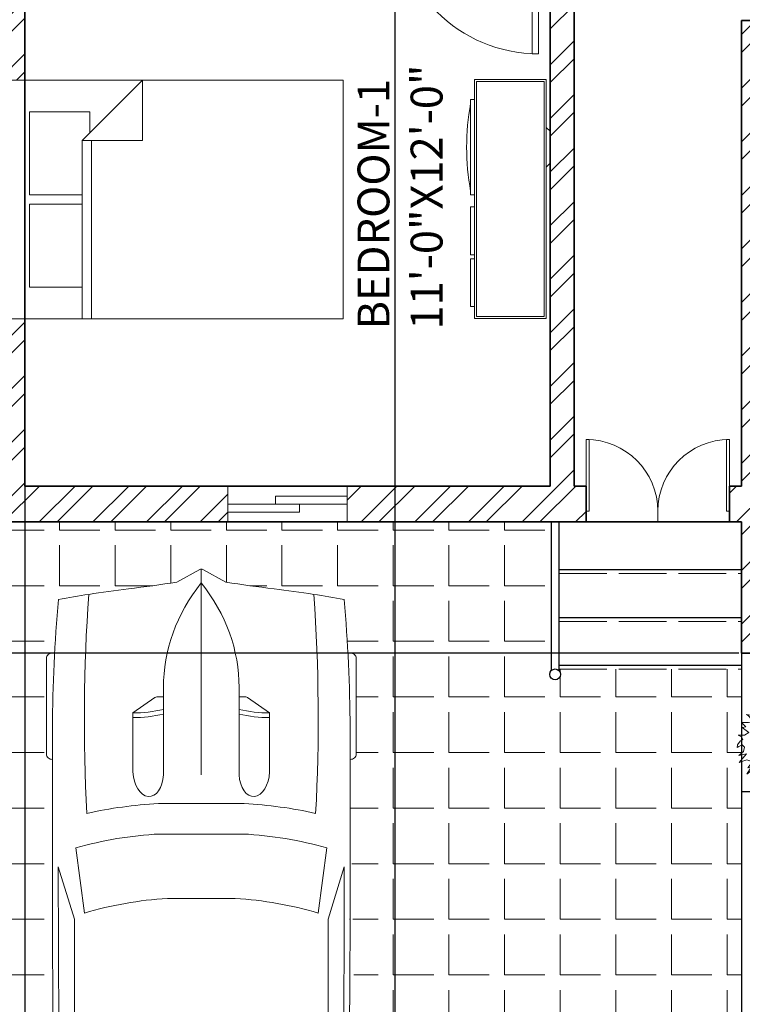
# Model space of a CAD drawing. Units: inches. Extents: x 889 to 1572, y 7262 to 8387.
# Tile 1 of 8: x 1024 to 1205, y 7495 to 7742. Entities that reach past the tile are written whole.
import ezdxf

# ---------------------------------------------------------------- set-up
doc = ezdxf.new("R2010")
doc.units = ezdxf.units.IN
doc.linetypes.add('ACAD_ISO02W100', pattern=[15, 12, -3])
for name, color, linetype, lineweight in [('A-ANNO-DIMS', 2, 'Continuous', 18), ('A-AREA-IDEN', 7, 'Continuous', 18), ('A-DOOR', 4, 'Continuous', 18), ('A-FLOR-STRS', 7, 'Continuous', 25), ('A-FURN', 8, 'Continuous', 18), ('A-STRS-HIDN', 8, 'ACAD_ISO02W100', 13), ('A-WALL', 7, 'Continuous', 35), ('A-WALL-PATT', 252, 'Continuous', 13), ('C-SITE', 7, 'Continuous', 30), ('C-VEHI', 8, 'Continuous', 18), ('L-PLNT', 94, 'Continuous', 13), ('L-PVMT-PATT', 252, 'Continuous', 13)]:
    doc.layers.add(name, color=color, linetype=linetype, lineweight=lineweight)
doc.layers.add('A-GLAZ', color=244, linetype='Continuous', lineweight=18, true_color=0x991b1e)
doc.styles.get("Standard").update_dxf_attribs({"font": 'arial.ttf'})
doc.dimstyles.new('ISO-25', dxfattribs={"dimtxt": 9, "dimasz": 2.5, "dimexe": 1.25, "dimexo": 0.625, "dimtad": 1, "dimlunit": 3, "dimtxsty": 'Standard', "dimcen": 2.5, "dimadec": 0, "dimazin": 0, "dimtfac": 1, "dimtmove": 0, "dimatfit": 3, "dimfxl": 1, "dimarcsym": 0})

# ---------------------------------------------------------------- blocks, each defined once
blk = doc.blocks.new('*U2')
for p, q in [((0, 0), (-1e-16, -5.999999999999999)), ((40, -6e-16), (40, -6))]:
    blk.add_line(p, q)
blk.add_lwpolyline([(0, 0), (5.6e-15, 40), (1.750000000000007, 40), (1.749999999999998, -7e-16)], close=True)
blk.add_arc((0, 0), 40, 0, 90)
blk = doc.blocks.new('*U3')
for p, q in [((0, 0), (0, -5.999999999999999)), ((-40, -6e-16), (-40, -6))]:
    blk.add_line(p, q)
blk.add_lwpolyline([(0, 0), (-7.1e-15, 40), (-1.750000000000007, 40), (-1.75, -7e-16)], close=True)
blk.add_arc((0, 0), 40, 90, 180)
blk = doc.blocks.new('*U5')
for p, q in [((-40, -1.47e-14), (-40, 5.999999999999984)), ((0, 0), (0, 5.999999999999999))]:
    blk.add_line(p, q)
blk.add_lwpolyline([(0, 0), (7.1e-15, -40), (-1.749999999999992, -40), (-1.75, -1e-16)], close=True)
blk.add_arc((0, 0), 40, 180, 270)
blk = doc.blocks.new('Bed - Queen')
for p, q in [((0, -80.00003000000002), (0, 0)), ((0, 0), (59.99998999999999, 0)), ((59.99998999999999, 0), (59.99998999999999, -80.00003000000002)), ((7.99999, -1.200000000000017), (28.79998, -1.200000000000017)), ((7.99999, -14.4), (7.99999, -1.200000000000017)), ((28.79998, -1.200000000000017), (28.79998, -14.4)), ((31.19999, -1.200000000000017), (51.99999000000001, -1.200000000000017)), ((31.19999, -14.4), (31.19999, -1.200000000000017)), ((51.99999000000001, -1.200000000000017), (51.99999000000001, -16.4)), ((0, -14.4), (44.79999999999999, -14.4)), ((59.99998999999999, -29.60000000000001), (44.79999999999999, -14.4)), ((44.79999999999999, -14.4), (44.79999999999999, -29.60000000000001)), ((44.79999999999999, -16.80000000000001), (0, -16.80000000000001)), ((51.99999000000001, -16.4), (46.79936, -16.4)), ((44.79999999999999, -29.60000000000001), (59.99998999999999, -29.60000000000001)), ((59.99998999999999, -80.00003000000002), (0, -80.00003000000002))]:
    blk.add_line(p, q)
blk = doc.blocks.new('Entertainment Center')
for p, q in [((-4, 0), (-5, -1)), ((4, 0), (-4, 0)), ((5, -1), (4, 0)), ((-17, -19.00000000000003), (-17, -1)), ((-17, -1), (43, -1)), ((-16.5, -18.50000000000003), (-16.5, -1.5)), ((-16.5, -1.5), (42.5, -1.5)), ((42.5, -1.5), (42.5, -18.50000000000003)), ((43, -1), (43, -19.00000000000003)), ((43, -19.00000000000003), (-17, -19.00000000000003)), ((42.5, -18.50000000000003), (-16.5, -18.50000000000003)), ((-12, -20.00000000000003), (-12, -19.00000000000003)), ((12, -19.00000000000003), (12, -20.00000000000003)), ((15, -20.00000000000003), (15, -19.00000000000003)), ((27, -19.00000000000003), (27, -20.00000000000003)), ((28, -20.00000000000003), (28, -19.00000000000003)), ((40, -19.00000000000003), (40, -20.00000000000003)), ((12, -20.00000000000003), (-12, -20.00000000000003)), ((27, -20.00000000000003), (15, -20.00000000000003)), ((40, -20.00000000000003), (28, -20.00000000000003))]:
    blk.add_line(p, q)
blk.add_arc((0, 40), 61.0000000000039, 259.6111000000045, 280.3888999999955)
blk = doc.blocks.new('*U19')
for points in [[(0, 60.6400000000001), (-3.051000000000385, 56.23799999999983), (-4.196000000000367, 52.81500000000005), (-5.33999999999969, 47.92499999999995), (-6.10299999999961, 45.96900000000005), (-11.0619999999999, 50.85899999999992), (-18.69100000000026, 52.32600000000002), (-20.98000000000002, 47.43600000000014), (-20.2170000000001, 43.52399999999988), (-20.5979999999995, 39.61100000000011), (-25.93899999999985, 43.03500000000008), (-27.84600000000001, 49.39200000000005), (-33.18600000000015, 52.32600000000002), (-30.51600000000008, 47.43600000000014), (-31.279, 43.03500000000008), (-30.13499999999976, 38.14400000000001), (-33.56799999999976, 35.21000000000004), (-40.8149999999996, 36.67700000000014), (-49.20799999999963, 38.14400000000001), (-46.91899999999987, 36.67700000000014), (-42.34100000000035, 31.78700000000004), (-42.34100000000035, 28.36400000000003), (-46.53699999999981, 27.38599999999997), (-55.69200000000001, 27.38599999999997), (-49.9699999999998, 22.00600000000008), (-54.54799999999977, 21.02799999999979), (-46.15599999999995, 14.67100000000005), (-51.4960000000001, 11.24799999999982), (-59.88799999999992, 11.24799999999982), (-55.69200000000001, 8.802999999999884), (-53.78499999999985, 5.380000000000109), (-57.21799999999984, 3.423000000000001), (-60.65100000000029, -1.467000000000098), (-61.0329999999999, -4.889999999999872), (-59.125, -3.422999999999774), (-54.54799999999977, -1.467000000000098), (-51.4960000000001, -4.401000000000067), (-53.02199999999993, -10.269), (-59.125, -15.16000000000008), (-49.20799999999963, -13.20399999999995), (-58.36200000000008, -24.45100000000002), (-48.44499999999971, -21.02799999999979), (-43.48600000000033, -22.49499999999989), (-43.10400000000027, -25.91799999999989), (-47.29999999999972, -31.29799999999978), (-43.10400000000027, -30.31999999999994), (-48.44499999999971, -39.61100000000011), (-38.52700000000004, -31.78700000000004), (-40.8149999999996, -36.18799999999988), (-32.42299999999977, -37.16599999999994), (-33.56799999999976, -43.52299999999991), (-35.47499999999991, -49.39200000000005), (-28.60899999999992, -44.99000000000001), (-23.64999999999964, -46.45700000000011), (-22.12400000000025, -51.83699999999999), (-21.74299999999949, -57.70499999999993), (-19.07299999999986, -52.32600000000002), (-15.63900000000012, -51.83699999999999), (-12.58799999999974, -58.68299999999976), (-11.0619999999999, -54.77099999999996), (-6.865999999999985, -49.39200000000005), (-6.865999999999985, -53.30399999999986), (-4.958999999999832, -48.41399999999999), (-1.907000000000152, -61.61700000000019), (-1.144000000000232, -51.34799999999995), (4.577999999999974, -59.17200000000002), (5.340999999999894, -54.28200000000015), (9.91800000000012, -56.72700000000009), (12.20700000000033, -60.63899999999989), (12.97000000000025, -47.92499999999995), (14.87700000000041, -44.50099999999998), (17.54700000000048, -47.43600000000014), (19.45500000000038, -52.81500000000005), (22.88799999999992, -60.63899999999989), (21.74299999999994, -49.39200000000005), (23.65000000000009, -46.45700000000011), (29.75399999999991, -47.92499999999995), (35.09400000000005, -52.32600000000002), (37.00099999999975, -53.79299999999989), (33.18700000000035, -46.45700000000011), (32.04200000000037, -41.567), (35.09400000000005, -39.12200000000007), (43.86799999999993, -40.58899999999994), (47.68200000000024, -42.05600000000004), (43.10500000000001, -36.18799999999988), (43.10500000000001, -33.74299999999994), (46.53800000000001, -31.29799999999978), (50.35200000000031, -32.76499999999987), (46.91899999999987, -26.40700000000015), (55.69300000000021, -22.49499999999989), (60.6520000000005, -22.98399999999992), (66.3739999999998, -22.00600000000008), (59.88899999999967, -20.04999999999995), (54.16700000000037, -18.09399999999982), (51.87800000000016, -15.64899999999989), (49.58899999999994, -12.22499999999991), (51.4970000000003, -10.269), (57.98099999999976, -9.779999999999973), (63.32200000000011, -7.335000000000036), (64.4659999999999, -2.933999999999969)], [(64.84799999999996, -2.933999999999969), (59.50700000000051, -5.378999999999905), (56.45600000000013, -4.401000000000067), (51.87800000000016, -2.444999999999936), (52.26000000000022, 0.9779999999998381), (55.31100000000015, 3.912000000000034), (59.88899999999967, 5.868999999999914), (62.94000000000005, 11.24799999999982), (58.36300000000028, 10.26999999999998), (54.54800000000023, 10.26999999999998), (51.11500000000024, 11.24799999999982), (53.7850000000003, 15.64899999999989), (57.98099999999976, 18.09400000000005), (60.6520000000005, 19.56100000000015), (56.07399999999961, 19.56100000000015), (51.11500000000024, 17.60500000000002), (46.53800000000001, 19.07200000000011), (46.15599999999995, 22.49600000000009), (49.58899999999994, 27.38599999999997), (52.26000000000022, 34.72100000000001), (49.58899999999994, 33.74299999999994), (44.24899999999979, 30.31999999999994), (41.19700000000011, 32.27600000000007), (41.57899999999972, 37.65499999999998), (43.86799999999993, 42.54600000000005), (43.10500000000001, 46.94700000000011), (40.05299999999988, 44.01299999999991), (36.23800000000028, 40.58899999999994), (33.56800000000021, 42.05700000000024), (33.95000000000027, 45.96900000000005), (35.47600000000012, 52.81500000000005), (31.2800000000002, 49.39200000000005), (26.70200000000022, 46.94700000000011), (28.22800000000007, 50.85899999999992), (28.60899999999992, 61.1289999999999), (24.79500000000007, 54.28200000000015), (18.69200000000046, 50.85899999999992), (17.92899999999963, 57.70600000000013), (12.97000000000025, 50.85899999999992), (7.248000000000047, 57.70600000000013), (5.340999999999894, 53.30399999999986), (0, 60.6400000000001)]]:
    blk.add_lwpolyline(points)
blk.add_lwpolyline([(0.3820000000005166, 1.95600000000013), (0, 0), (1.907000000000152, 0.4890000000000328), (2.288999999999759, 1.467000000000098)], close=True)
blk = doc.blocks.new('*U21')
for p, q in [((21.10406751471477, 37.40863046792069), (21.10406751471477, 36.83230215753705)), ((46.55368679439944, 38.88847654282876), (22.35054758993934, 38.88847654282876)), ((47.80016686962392, 37.39011648242055), (47.80016686962392, 37.40863046792069)), ((135.4513231603356, 37.07354110333037), (135.4513231603356, 37.40863046792069)), ((136.6978032355602, 38.88847654282876), (160.90094244002, 38.88847654282867)), ((162.1474225152445, 37.40863046792049), (162.1474225152445, 36.77402019194128)), ((87.98532186932616, 31.87120872459877), (74.75900729854769, 35.92175679182955)), ((134.313356548143, 35.6043097713567), (119.2882629232503, 31.77757799177584)), ((186.4728846989705, -33.49860931502491), (186.4728846989718, 33.49860931502465)), ((188.3990091454065, -32.75868627757393), (188.3990091454077, 32.75868627757058)), ((70.0302824853563, 31.53613089391356), (86.40615155322342, 29.35124891408057)), ((138.4228833961707, 29.35124891408074), (157.2465674415997, 29.35124891408074)), ((186.4728846989718, 29.35124891408083), (167.0083537481071, 29.35124891408083)), ((164.515393597658, 26.39155676426461), (164.5153935976578, -26.39155676426503)), ((32.26591480791686, 11.62530558863241), (36.12873726252356, 17.16961494239206)), ((36.12873726252356, 17.16961494239206), (50.93891189819171, 17.16961494239206)), ((32.12291633764599, 9.505833383620029), (32.12291633764599, 11.15369945057711)), ((58.9167604809788, -10.77488335095668), (58.9167604809788, 10.77488335095617)), ((66.55009204259746, -10.5288681329018), (66.55009204259746, 10.52886813290129)), ((186.4728846989718, -10.5288681329018), (186.4728846989718, 10.52886813290129)), ((29.77279020470884, 9.505833383620029), (51.68362801571248, 9.505833383620029)), ((82.73706193978568, 8.496039918672748), (82.73706193978568, -8.49603991867258)), ((3.266462181856987, 6.128290093440767), (0.1022408397004821, 0.4060708604429806)), ((-4.43e-14, -2.558e-13), (51.68362801571248, -2.558e-13)), ((0.1022408397004821, -0.4060708604432933), (3.266462181856987, -6.128290093441194)), ((29.77279020470884, -9.50583338362054), (51.68362801571248, -9.50583338362054)), ((32.12291633764599, -9.50583338362054), (32.12291633764599, -11.15369945057762)), ((32.26591480791686, -11.62530558863292), (36.12873726252356, -17.16961494239257)), ((36.12873726252356, -17.16961494239257), (50.93891189819171, -17.16961494239257)), ((86.40615155322318, -29.35124891408145), (70.03028248535594, -31.53613089391442)), ((157.2465674415997, -29.35124891408117), (138.4228833961707, -29.35124891408126)), ((167.008353748107, -29.35124891408126), (186.4728846989707, -29.35124891408108)), ((87.98532186932607, -31.87120872459903), (74.7590072985476, -35.92175679182964)), ((134.3133565481428, -35.60430977135721), (119.2882629232503, -31.77757799177618)), ((21.10406751471477, -37.4086304679212), (21.10406751471477, -36.83230215753756)), ((135.4513231603355, -37.07354110333088), (135.4513231603355, -37.4086304679212)), ((162.1474225152445, -37.408630467921), (162.1474225152445, -36.77402019194179)), ((46.55368679439944, -38.88847654282927), (22.35054758993934, -38.88847654282927)), ((47.80016686962392, -37.39011648242107), (47.80016686962392, -37.4086304679212)), ((136.6978032355602, -38.88847654282927), (160.9009424400199, -38.88847654282918))]:
    blk.add_line(p, q)
for centre, major_axis, ratio, start_param, end_param in [((41.19115208863305, -490.8631038926156), (1.294e-13, 528.2339998381949), 0.8423038695439741, 0.0028100083536837, 0.0755983031096952), ((22.35054758993934, 37.40863046792072), (2.08e-14, -1.479846074908118), 0.842303869543976, 3.141592653589776, 4.712388980384677), ((64.48199294511879, -10555.61767587835), (1.907644e-10, 10593.02630634627), 0.842303869543847, -0.0133969486112073, 0.0027970409639888), ((46.55368679439944, 37.40863046792072), (2.2e-14, 1.479846074908118), 0.8423038695439758, -1.570796326794884, 1.73e-14), ((136.6978032355602, 37.40863046792072), (2.357e-13, -1.479846074908118), 0.842303869543976, 3.141592653589603, 4.712388980384554), ((160.90094244002, 37.40863046792052), (5.59e-14, 1.479846074908118), 0.842303869543976, -1.570796326794865, 4.44e-14), ((180.6280394947615, 35.8381667808375), (7.4e-14, 2.219769112362114), 0.8423038695439693, -0.0130174256259048, 1.249894140392862), ((64.48199294754608, -10556.35759891604), (1.349839377e-06, 10595.3130398087), 0.8423038681351469, -0.0133969484821159, -0.0130174254969711), ((183.9799245485216, 32.75868627756583), (8.56e-14, -5.246425615115243), 0.8423038695439737, 1.570796326795794, 3.128195704978164), ((266.0300214172791, -27.52442688366631), (1.966072e-10, 313.3077612809058), 0.8423038695435284, 1.367075990158062, 1.391760499156098), ((64.4819929449925, -10555.61767590795), (1.9177683e-09, -10591.54646030096), 0.8423038695482963, 3.133765086725325, 3.140440689641252), ((183.9799245485226, 33.49860931502124), (3e-16, -2.959692149816168), 0.8423038695439952, 1.570796326796048, 3.128195704978389), ((37.47375371777758, -593.9621830607928), (6.21e-14, -623.32820996736), 0.8423038695439826, 3.09604606856106, 3.200911180495224), ((135.2911776514449, 5.387441675478555), (2.2715e-12, 81.77258453065997), 0.8423038695439563, 1.245306111696802, 1.507880129813836), ((95.78879860270445, -3666.353346297651), (1.949864e-10, -3698.236159209632), 0.8423038695446962, 3.134048706297306, 3.14409775411291), ((259.1750197310735, -27.52442688366614), (1.506617e-10, -305.3028914627677), 0.8423038695443789, 4.528606069860317, 4.561837674556238), ((134.4003789125686, 5.387441675477674), (4.276e-13, -89.7774543484738), 0.84230386954398, 4.44948196380473, 4.652344057257214), ((149.595361812917, 2.799442537139299), (8.561e-13, -79.57966406425402), 0.842303869543983, 4.372215489277867, 4.640744122441986), ((17.08207736189386, -1.421e-13), (6.87e-14, 147.0179238898305), 0.8423038695439764, 4.511394369635731, 4.913383591133647), ((35.90576140732288, -1.421e-13), (6.87e-14, 147.0179238898305), 0.8423038695439764, 4.511394369635731, 4.913383591133647), ((167.0083537481071, 26.39155676426464), (1.394e-13, 2.959692149816236), 0.842303869543976, 5.55e-14, 1.57079632679492), ((-204.4946649195746, 52.39684969293512), (4.12053e-11, -250.9602162198571), 0.8423038695441164, 1.385369446298923, 1.434372047871027), ((13.03653510440275, 17.00972444508943), (1.2303e-12, 27.41599049210566), 0.8423038695439277, 4.435146050259648, 4.718221029521873), ((14.20086229321332, 17.00972444508943), (1.2303e-12, 27.41599049210566), 0.8423038695439277, 4.435146050259648, 4.718221029521873), ((50.7902773840875, 13.33772416300607), (6.340077547122382, -0.356608581037027), 0.6038335755719145, -1.39555193967809, 1.581314658479915), ((32.74615637525823, 11.15369945057713), (1.313e-13, 0.7399230374541176), 0.8423038695439091, 0.8797135699495516, 1.570796326795045), ((29.77279020470884, -46.66302566589627), (5.12e-14, 56.16885904951626), 0.842303869543976, 7e-16, 0.5903187773915901), ((0.6232400376122422, -1.421e-13), (1e-16, -0.7399230374541245), 0.842303869543842, 4.131459131953847, 5.293318828815531), ((29.77279020470884, 46.66302566589578), (4.004e-13, 56.16885904951626), 0.8423038695439734, 2.55127387619821, 3.141592653589801), ((-204.4946649195746, -52.39684969293552), (4.02945e-11, 250.9602162198562), 0.8423038695441192, -1.43437204787103, -1.385369446298926), ((13.03653510440275, -17.00972444508983), (1.2568e-12, -27.41599049210552), 0.8423038695439318, 1.564964277657711, 1.848039256919935), ((14.20086229321332, -17.00972444508983), (1.2568e-12, -27.41599049210552), 0.8423038695439318, 1.564964277657711, 1.848039256919935), ((149.5953618129329, -2.799442537137565), (4.0897e-12, -79.57966406427697), 0.8423038695439419, -1.499151468852248, -1.230622835688196), ((32.74615637525823, -11.1536994505777), (1.3e-13, -0.7399230374541176), 0.8423038695439093, 4.712388980384541, 5.403471737230034), ((134.4003789125684, -5.387441675478584), (4.2949e-12, -89.77745434847827), 0.8423038695439354, -1.510751403667474, -1.307889310215002), ((135.2911776514465, -5.387441675480715), (3.2038e-12, -81.77258453066244), 0.8423038695439492, -1.50788012981387, -1.245306111696839), ((259.1750197310694, 27.52442688365929), (1.08535e-11, 305.3028914629043), 0.8423038695439974, 1.721347632622872, 1.754579237318777), ((167.008353748107, -26.39155676426503), (1.02e-14, -2.959692149816192), 0.8423038695439885, 4.712388980384686, 6.283185307179581), ((266.0300214172791, 27.52442688366566), (8.75241e-11, 313.3077612806533), 0.8423038695441819, 1.749832154434603, 1.774516663432659), ((37.47375371777847, 593.9621830607904), (1.1693e-12, -623.3282099673584), 0.8423038695439528, -0.0593185269054384, 0.0455465850287298), ((95.78879860271888, 3666.35334629765), (1.637818e-10, -3698.236159209629), 0.8423038695447546, -0.0025051005232382, 0.007543947292366), ((183.9799245485216, -33.4986093150211), (9.3e-15, 2.959692149816141), 0.8423038695439732, 3.154989602201626, 4.71238898038339), ((183.9799245485177, -32.7586862775633), (2.428e-13, -5.246425615118353), 0.8423038695439808, 0.0133969486110846, 1.570796326792831), ((41.19115208863322, 490.8631038926152), (1.37757e-11, -528.2339998381949), 0.8423038695440652, -0.0755983031097181, -0.0028100083537155), ((64.48199294495228, 10555.61767590795), (6.117947e-10, 10593.02630637587), 0.8423038695458146, 3.138795612625926, 3.154989602201039), ((64.48199294503607, 10555.61767590793), (1.6049794e-09, -10591.54646030094), 0.8423038695397146, 0.0011519639481523, 0.0078275668641468), ((180.6280394947581, -35.83816678083949), (2.274e-13, -2.219769112363032), 0.8423038695439803, -1.249894138785958, 0.0130174256254374), ((22.35054758993934, -37.40863046792117), (2.2e-14, 1.479846074908118), 0.8423038695439758, 1.570796326794908, 3.14159265358981), ((46.55368679439944, -37.40863046792117), (2.08e-14, -1.479846074908118), 0.842303869543976, -1.69e-14, 1.570796326794884), ((136.6978032355602, -37.40863046792109), (1.56e-14, -1.479846074908162), 0.8423038695440105, -1.570796326794875, -1.27e-14), ((160.9009424400199, -37.408630467921), (1.969e-13, 1.479846074908162), 0.8423038695440109, 3.141592653589951, 4.712388980384771), ((64.48199294197605, 10556.3575989598), (9.365289701e-07, 10595.31303985772), 0.8423038705260315, 3.154610079306566, 3.154989602290631)]:
    blk.add_ellipse(centre, major_axis=major_axis, ratio=ratio, start_param=start_param, end_param=end_param)
at = {"extrusion": (0, 0, -1)}
blk.add_ellipse((50.7902773840875, -13.33772416300655), major_axis=(6.340077547122382, 0.3566085810370246), ratio=0.6038335755719145, start_param=-1.39555193967809, end_param=1.581314658479915, dxfattribs=at)
blk = doc.blocks.new('GLAZ-SLIDER-30IN')
for p, q in [((0.0001447784702577, 29.99977559742911), (0.0001447784702577, 11.9997755974291)), ((2.000144778470257, 29.99977559742911), (2.000144778470257, -0.0002244025708933)), ((4.000144778470257, 17.99977559742911), (2.000144778470257, 17.99977559742911)), ((4.000144778470257, 17.99977559742911), (4.000144778470257, -0.0002244025708933)), ((2.000144778470257, 11.9997755974291), (0.0001447784702577, 11.9997755974291))]:
    blk.add_line(p, q)
blk = doc.blocks.new('*D69')
at = {"layer": 'A-ANNO-DIMS', "color": 0, "lineweight": -2, "transparency": 16777216}
for p, q in [((1016.048608, 7615.106231), (1016.048608, 7262.354215000001)), ((1436.048608, 7582.106231), (1436.048608, 7262.354215000001)), ((1018.548608, 7263.604215), (1433.548608, 7263.604215))]:
    blk.add_line(p, q, dxfattribs=at)
at = {"layer": 'A-ANNO-DIMS', "color": 0, "transparency": 16777216}
for points in [[(1018.548608, 7264.020881666667), (1018.548608, 7263.187548333333), (1016.048608, 7263.604215)], [(1433.548608, 7264.020881666667), (1433.548608, 7263.187548333333), (1436.048608, 7263.604215)]]:
    blk.add_solid(points, dxfattribs=at)
at = {"layer": 'Defpoints', "color": 0, "transparency": 16777216}
for p in [(1016.048608, 7615.731230999999), (1436.048608, 7582.731231), (1436.048608, 7263.604215)]:
    blk.add_point(p, dxfattribs=at)
at = {"layer": 'A-ANNO-DIMS', "color": 0, "transparency": 16777216, "insert": (1226.048608, 7268.827441466576), "char_height": 9, "attachment_point": 5}
blk.add_mtext('35\'-0"', dxfattribs=at)
blk = doc.blocks.new('*D72')
at = {"layer": 'A-ANNO-DIMS', "color": 0, "lineweight": -2, "transparency": 16777216}
for p, q in [((1204.423608, 7615.731231000004), (932.7986080000009, 7615.731231000004)), ((934.0486080000009, 7585.231231000003), (934.0486080000009, 7613.231231000003)), ((1204.423608, 7582.731231000003), (932.7986080000009, 7582.731231000003))]:
    blk.add_line(p, q, dxfattribs=at)
at = {"layer": 'A-ANNO-DIMS', "color": 0, "transparency": 16777216}
for points in [[(933.6319413333342, 7613.231231000003), (934.4652746666675, 7613.231231000003), (934.0486080000009, 7615.731231000004)], [(933.6319413333342, 7585.231231000003), (934.4652746666675, 7585.231231000003), (934.0486080000009, 7582.731231000003)]]:
    blk.add_solid(points, dxfattribs=at)
at = {"layer": 'Defpoints', "color": 0, "transparency": 16777216}
for p in [(934.0486080000009, 7615.731231000004), (1205.048608, 7615.731231000004), (1205.048608, 7582.731231000003)]:
    blk.add_point(p, dxfattribs=at)
at = {"layer": 'A-ANNO-DIMS', "color": 0, "transparency": 16777216, "insert": (928.8284511105074, 7599.231231000001), "char_height": 9, "attachment_point": 5, "rotation": 90}
blk.add_mtext('2\'-9"', dxfattribs=at)
blk = doc.blocks.new('*D76')
at = {"layer": 'A-ANNO-DIMS', "color": 0, "lineweight": -2, "transparency": 16777216}
for p, q in [((1025.048608, 7774.106231000001), (1025.048608, 7262.354215000001)), ((1118.048608, 7774.106231000001), (1118.048608, 7262.354215000001)), ((1027.548608, 7263.604215), (1115.548608, 7263.604215))]:
    blk.add_line(p, q, dxfattribs=at)
at = {"layer": 'A-ANNO-DIMS', "color": 0, "transparency": 16777216}
for points in [[(1027.548608, 7264.020881666667), (1027.548608, 7263.187548333333), (1025.048608, 7263.604215)], [(1115.548608, 7264.020881666667), (1115.548608, 7263.187548333333), (1118.048608, 7263.604215)]]:
    blk.add_solid(points, dxfattribs=at)
at = {"layer": 'Defpoints', "color": 0, "transparency": 16777216}
for p in [(1025.048608, 7774.731231), (1118.048608, 7774.731231), (1118.048608, 7263.604215)]:
    blk.add_point(p, dxfattribs=at)
at = {"layer": 'A-ANNO-DIMS', "color": 0, "transparency": 16777216, "insert": (1071.548608, 7268.824371889495), "char_height": 9, "attachment_point": 5}
blk.add_mtext('7\'-9"', dxfattribs=at)

msp = doc.modelspace()

# ---------------------------------------------------------------- hatches: boundary and pattern name
at = {"layer": 'A-WALL-PATT'}
h = msp.add_hatch(dxfattribs=at)
h.set_pattern_fill('ANSI32', color=256)
h.set_pattern_definition([(45, (0, 0), (-6.735192090801866, 6.735192090801866), []), (45, (4.49013, 0), (-6.735192090801866, 6.735192090801866), [])])
h.paths.add_polyline_path([(1166.048608413352, 7624.731230872604), (1163.048608413352, 7624.731230872604), (1163.048608413352, 7774.731230872602), (1154.048608413352, 7774.731230872602), (1154.048608413352, 7768.731230872603), (1157.048608413352, 7768.731230872603), (1157.048608413352, 7624.731230872604), (1106.048608413347, 7624.731230872605), (1106.048608413347, 7615.731230872604), (1166.048608413352, 7615.731230872604), (1166.048608413352, 7618.431230872605)])
h.paths.add_polyline_path([(1025.048608413352, 7666.731230872606), (1016.048608413352, 7666.731230872606), (1016.048608413352, 7615.731230872608), (1076.048608413347, 7615.731230872606), (1076.048608413347, 7624.731230872605), (1025.048608413352, 7624.731230872606)])
h.paths.add_polyline_path([(1025.048608413352, 7768.731230872607), (1118.048608413352, 7768.731230872605), (1118.048608413352, 7774.731230872603), (1025.048608413352, 7774.731230872607), (1025.048608413352, 7897.731230872607), (1115.048608413351, 7897.731230872603), (1115.048608413351, 7906.731230872605), (1109.048608413352, 7906.731230872605), (1109.048608413352, 7903.731230872605), (1025.048608413352, 7903.731230872607), (1025.048608413352, 7923.231230872606), (1016.048608413352, 7923.231230872606), (1016.048608413352, 7726.731230872608), (1025.048608413352, 7726.731230872608)])
h.paths.add_polyline_path([(1436.048608413352, 7897.731230872607), (1427.048608413351, 7897.731230872607), (1427.048608413351, 7883.37377559743), (1436.048608413352, 7883.37377559743)])
h.paths.add_polyline_path([(1436.048608413352, 7853.373775597429), (1427.048608413351, 7853.373775597429), (1427.048608413351, 7843.731230872608), (1415.048608413352, 7843.731230872608), (1415.048608413352, 7837.731230872607), (1427.048608413351, 7837.731230872607), (1427.048608413351, 7831.731230872607), (1436.048608413352, 7831.731230872607)])
h.paths.add_polyline_path([(1436.048608413352, 8010.183478752281), (1427.048608413351, 8010.183478752281), (1427.048608413351, 7970.456226002662), (1370.048608413352, 7970.456226002662), (1370.048608413352, 7963.731230872607), (1427.048608413351, 7963.731230872608), (1427.048608413351, 7957.731230872607), (1436.048608413352, 7957.731230872607)])
h.paths.add_polyline_path([(1436.048608413352, 7747.731230872607), (1427.048608413352, 7747.731230872607), (1427.048608413352, 7741.731230872608), (1344.721387503392, 7741.731230872608), (1344.721387503392, 7735.731230872609), (1349.048608413352, 7735.731230872609), (1349.048608413352, 7672.731230872607), (1355.048608413352, 7672.731230872606), (1355.048608413352, 7735.731230872609), (1427.048608413352, 7735.731230872608), (1427.048608413352, 7721.931475650177), (1436.048608413352, 7721.931475650177)])
h.paths.add_polyline_path([(1436.048608413352, 7700.931475650178), (1427.048608413352, 7700.931475650178), (1427.048608413352, 7591.731230872608), (1355.048608413352, 7591.731230872608), (1355.048608413352, 7642.731230872605), (1349.048608413352, 7642.731230872607), (1349.048608413352, 7591.731230872608), (1310.048608413352, 7591.731230872608), (1310.048608413352, 7582.731230872609), (1436.048608413352, 7582.731230872608)])
h.paths.add_polyline_path([(1392.41988820942, 8272.731230872607), (1331.048608413352, 8272.731230872607), (1331.048608413352, 8263.731230872607), (1349.048608413352, 8263.731230872607), (1349.048608413352, 8224.731230872603), (1355.048608413352, 8224.731230872607), (1355.048608413352, 8263.731230872607), (1392.41988820942, 8263.731230872607)])
h.paths.add_polyline_path([(1271.048608413352, 8272.731230872607), (1196.736043973615, 8272.731230872607), (1196.736043973615, 8263.731230872607), (1247.048608413352, 8263.731230872607), (1247.048608413352, 8203.731230872605), (1244.048608413352, 8203.731230872605), (1244.048608413352, 8197.731230872605), (1247.048608413352, 8197.731230872605), (1247.048608413353, 8161.731230872605), (1253.048608413352, 8161.731230872605), (1253.048608413352, 8185.731230872605), (1295.048608413353, 8185.731230872603), (1295.048608413353, 8191.731230872607), (1253.048608413352, 8191.731230872605), (1253.048608413352, 8263.731230872607), (1271.048608413352, 8263.731230872607)])
h.paths.add_polyline_path([(1175.736043973615, 8272.731230872607), (1102.037311183427, 8272.731230872607), (1102.037311183427, 8263.731230872607), (1157.048608413352, 8263.731230872607), (1157.048608413352, 8158.731230872607), (1163.048608413352, 8158.731230872607), (1163.048608413352, 8197.731230872605), (1214.048608413352, 8197.731230872605), (1214.048608413352, 8203.731230872605), (1163.048608413352, 8203.731230872605), (1163.048608413352, 8263.731230872607), (1175.736043973615, 8263.731230872607)])
h.paths.add_polyline_path([(1072.037311183427, 8272.731230872607), (1016.048608413352, 8272.731230872607), (1016.048608413352, 8221.731230872607), (1025.048608413352, 8221.731230872607), (1025.048608413352, 8263.731230872607), (1072.037311183427, 8263.731230872607)])
h.paths.add_polyline_path([(1163.048608413352, 8122.731230872608), (1157.048608413352, 8122.731230872608), (1157.048608413352, 8119.731230872607), (1025.048608413352, 8119.731230872607), (1025.048608413352, 8161.731230872607), (1016.048608413352, 8161.731230872607), (1016.048608413352, 8071.731230872606), (1025.048608413352, 8071.731230872606), (1025.048608413352, 8113.731230872607), (1157.048608413352, 8113.731230872607), (1157.048608413352, 8110.731230872607), (1163.048608413352, 8110.731230872607)])
h.paths.add_polyline_path([(1025.048608413352, 8011.731230872607), (1016.048608413352, 8011.731230872607), (1016.048608413352, 7944.231230872607), (1025.048608413352, 7944.231230872607), (1025.048608413352, 7963.731230872607), (1109.048608413352, 7963.731230872605), (1109.048608413352, 7936.731230872606), (1115.048608413351, 7936.731230872606), (1115.048608413351, 7963.731230872605), (1163.048608413352, 7963.731230872607), (1163.048608413352, 8074.731230872606), (1157.048608413352, 8074.731230872606), (1157.048608413352, 7969.731230872607), (1025.048608413352, 7969.731230872607)])
h.paths.add_polyline_path([(1314.721387503392, 7741.731230872608), (1307.048608413352, 7741.731230872608), (1307.048608413352, 7837.731230872609), (1319.048608413352, 7837.731230872609), (1319.048608413352, 7843.731230872608), (1307.048608413352, 7843.731230872608), (1307.048608413352, 7963.731230872608), (1310.048608413352, 7963.731230872607), (1310.048608413352, 7970.456226002662), (1301.048608413352, 7970.456226002662), (1301.048608413352, 7837.731230872607), (1301.048608413352, 7741.731230872608), (1250.048608413352, 7741.731230872608), (1250.048608413352, 7735.731230872609), (1314.721387503392, 7735.731230872609)])
h.paths.add_polyline_path([(1211.048608413352, 7735.731230872609), (1214.048608413352, 7735.731230872609), (1214.048608413352, 7741.731230872608), (1205.048608413352, 7741.731230872608), (1205.048608413352, 7624.731230872601), (1202.048608413352, 7624.731230872602), (1202.048608413352, 7615.731230872603), (1205.048608413352, 7615.731230872604), (1205.048608413352, 7582.731230872609), (1250.048608413353, 7582.731230872609), (1250.048608413353, 7591.73123087261), (1211.048608413352, 7591.731230872611)])
h.paths.add_polyline_path([(1436.048608413352, 8260.718366180157), (1427.048608413352, 8260.718366180157), (1427.048608413351, 8191.731230872607), (1355.048608413352, 8191.731230872607), (1355.048608413352, 8194.731230872607), (1349.048608413352, 8194.731230872603), (1349.048608413352, 8191.731230872607), (1343.048608413353, 8191.731230872607), (1343.048608413353, 8185.731230872608), (1427.048608413352, 8185.731230872608), (1427.048608413351, 8070.183478752282), (1436.048608413352, 8070.183478752282)])
at = {"layer": 'L-PVMT-PATT'}
h = msp.add_hatch(dxfattribs=at)
h.set_pattern_fill('ANGLE', color=256, scale=2)
h.set_pattern_definition([(0, (0, 0), (0, 13.97), [10.16, -3.81]), (90, (0, 0), (-13.97, 9e-16), [10.16, -3.81])])
h.paths.add_polyline_path([(1205.048608413351, 7555.446171834415), (1204.522810014118, 7555.264684699134), (1205.048608413351, 7555.910703335377), (1205.048608413352, 7557.193763035785), (1204.375295363129, 7557.060960744141), (1205.048608413352, 7557.600559978721), (1205.048608413352, 7559.617877481), (1204.375295363129, 7559.330134346581), (1204.006412068125, 7559.046511813157), (1204.08026606115, 7559.708297724476), (1205.048608413352, 7561.087614386948), (1205.048608413352, 7561.676628270497), (1205.03901462505, 7561.693848793495), (1204.227780712139, 7562.166553015865), (1205.048608413352, 7562.166553015865), (1205.048608413352, 7565.277573844389), (1205.03901462505, 7565.286594218571), (1205.048608413352, 7565.286594218571), (1205.048608413352, 7578.731230872603), (1159.234402724352, 7578.731230872605), (1159.234402724352, 7578.363210835082, -0.1960004452144572), (1159.622195581334, 7577.411949376209, -1.441243748687975), (1157.234402724352, 7578.304265881411), (1157.234402724352, 7615.731230872604), (1016.048608413352, 7615.731230872608), (1016.048608413352, 7399.731230872607), (1022.048608413351, 7399.731230872605), (1205.048608413347, 7399.731230872603), (1205.048608413347, 7402.731230872603)])
edge = h.paths.add_edge_path(flags=16)
edge.add_ellipse((-9486.215667076898, 7539.371191098851), major_axis=(10593.02630634627, 3.017206e-10), ratio=0.8423038695454096, start_angle=-0.38386677879407216, end_angle=0.09022908859270728, ccw=False)
edge.add_ellipse((1106.81063926937, 7467.155380808408), major_axis=(1.479846074908209, 2.4527e-12), ratio=0.8423038695436039, start_angle=-9.487166607868858e-11, end_angle=89.99999999990501, ccw=False)
edge.add_line((1108.290485344278, 7467.155380808408), (1108.290485344278, 7442.952241603949))
edge.add_ellipse((1106.81063926937, 7442.952241603949), major_axis=(-1.479846074908209, 2.4527e-12), ratio=0.8423038695436041, start_angle=90.00000000009499, end_angle=180.0000000000949, ccw=False)
edge.add_line((1106.81063926937, 7441.705761528725), (1106.176028993391, 7441.705761528725))
edge.add_ellipse((-9486.215667076898, 7539.371191098851), major_axis=(10593.02630634627, 3.017206e-10), ratio=0.8423038695454096, start_angle=-0.6186431963208179, end_angle=-0.5282714718196075, ccw=False)
edge.add_ellipse((1105.240175582287, 7423.225144549206), major_axis=(2.219769112362271, 3.512e-12), ratio=0.8423038695437586, start_angle=-0.6282372162759771, end_angle=68.464756600913, ccw=False)
edge.add_ellipse((-9486.955590114589, 7539.371191096425), major_axis=(-10595.31303979869, 5.7334850558e-06), ratio=0.8423038635969176, start_angle=179.3534459339559, end_angle=179.3717628147891, ccw=False)
edge.add_ellipse((1102.160695079015, 7419.873259495446), major_axis=(-5.246425615115091, 6.131e-13), ratio=0.8423038695439657, start_angle=90.00000000006861, end_angle=179.3534459029308, ccw=False)
edge.add_line((1102.16069507902, 7415.45417489856), (1036.643322523875, 7415.454174898562))
edge.add_ellipse((1036.643322523886, 7419.87325949545), major_axis=(5.246425615118246, 3.3658e-12), ratio=0.8423038695439792, start_angle=180.6465540970289, end_angle=269.9999999998247, ccw=False)
edge.add_ellipse((11625.75960776125, 7539.371191101991), major_axis=(-10595.31303986147, 2.5904085676e-06), ratio=0.8423038722500887, start_angle=0.6282372302511021, end_angle=0.6465541110841855, ccw=False)
edge.add_ellipse((1033.56384202061, 7423.225144549211), major_axis=(2.219769112362928, 1.9515e-12), ratio=0.8423038695441785, start_angle=111.5352435039708, end_angle=180.6282372161348, ccw=False)
edge.add_ellipse((11625.0196847094, 7539.371191099013), major_axis=(-10593.02630637587, 5.863276e-10), ratio=0.8423038695454017, start_angle=0.528271471820517, end_angle=0.646554097064211, ccw=False)
edge.add_line((1032.627988609511, 7441.705761528725), (1031.993378333528, 7441.705761528725))
edge.add_ellipse((1031.993378333528, 7442.952241603949), major_axis=(1.479846074908209, 2.4527e-12), ratio=0.8423038695436039, start_angle=179.999999999905, end_angle=269.999999999905, ccw=False)
edge.add_line((1030.51353225862, 7442.952241603949), (1030.51353225862, 7467.155380808408))
edge.add_ellipse((1031.993378333528, 7467.155380808408), major_axis=(-1.479846074908209, 2.4527e-12), ratio=0.8423038695436041, start_angle=-89.99999999990501, end_angle=9.498535291641019e-11, ccw=False)
edge.add_ellipse((11625.0196847094, 7539.371191099013), major_axis=(-10593.02630637587, 5.863276e-10), ratio=0.8423038695454017, start_angle=-0.0902290885899788, end_angle=0.38386677879549325, ccw=False)
edge.add_ellipse((1031.993378333528, 7557.299497249569), major_axis=(-1.479846074907982, 9.504e-13), ratio=0.8423038695443477, start_angle=3.6777692002942786e-11, end_angle=90.00000000003672, ccw=False)
edge.add_line((1030.51353225862, 7557.299497249569), (1030.51353225862, 7581.502636454029))
edge.add_ellipse((1031.993378333528, 7581.502636454029), major_axis=(-1.479846074907982, 2.1793e-12), ratio=0.8423038695437334, start_angle=-89.99999999991559, end_angle=8.44124770082999e-11, ccw=False)
edge.add_line((1031.993378333528, 7582.749116529253), (1032.569706643912, 7582.749116529253))
edge.add_ellipse((1560.265112694065, 7562.662031955335), major_axis=(528.2339998381949, 5.3105e-12), ratio=0.8423038695440039, start_angle=176.3495724143003, end_angle=177.8200496863542, ccw=False)
edge.add_ellipse((1096.926435685115, 7337.82316262669), major_axis=(-313.3077612789123, 2.032944e-09), ratio=0.84230386954869, start_angle=-77.87403444734417, end_angle=-76.21947101013029, ccw=False)
edge.add_ellipse((1096.926435685109, 7344.678164312899), major_axis=(-305.3028914625973, 2.877231e-10), ratio=0.842303869544824, start_angle=-79.79046100280272, end_angle=-77.55537270650188, ccw=False)
edge.add_ellipse((1017.005159108514, 7808.347848963542), major_axis=(250.9602162202823, 3.689106e-10), ratio=0.8423038695427255, start_angle=-80.7434339928827, end_angle=-77.44506735594696)
edge.add_line((1063.273718708008, 7600.586721862112), (1069.402008801449, 7603.975488617634))
edge.add_line((1069.402008801449, 7603.975488617634), (1075.53029889489, 7600.586721862112))
edge.add_ellipse((1121.798858494384, 7808.347848963542), major_axis=(-250.9602162202835, 3.684091e-10), ratio=0.8423038695427219, start_angle=77.44506735594675, end_angle=80.74343399288247)
edge.add_ellipse((1041.877581917783, 7344.678164312894), major_axis=(305.3028914626093, 3.003322e-10), ratio=0.842303869544806, start_angle=77.55537270649842, end_angle=79.79046100279919, ccw=False)
edge.add_ellipse((1041.877581917783, 7337.82316262669), major_axis=(313.3077612789065, 2.0431705e-09), ratio=0.8423038695487045, start_angle=76.21947101012842, end_angle=77.87403444734218, ccw=False)
edge.add_ellipse((578.5389049088338, 7562.662031955335), major_axis=(-528.2339998381949, 1.51629e-11), ratio=0.8423038695441082, start_angle=182.1799503136469, end_angle=183.6504275857008, ccw=False)
edge.add_line((1106.234310958986, 7582.749116529253), (1106.81063926937, 7582.749116529253))
edge.add_ellipse((1106.81063926937, 7581.502636454029), major_axis=(1.479846074908209, 2.4524e-12), ratio=0.8423038695436039, start_angle=-9.487166607868858e-11, end_angle=89.99999999989461, ccw=False)
edge.add_line((1108.290485344278, 7581.502636454029), (1108.290485344278, 7557.299497249569))
edge.add_ellipse((1106.81063926937, 7557.299497249569), major_axis=(1.479846074908209, 6.78e-13), ratio=0.8423038695442183, start_angle=269.99999999997374, end_angle=359.9999999999738, ccw=False)
edge = h.paths.add_edge_path(flags=0)
edge.add_ellipse((-9486.215667106499, 7539.371191098978), major_axis=(10591.54646030096, 1.2635629e-09), ratio=0.8423038695462665, start_angle=-0.3777641939166756, end_angle=-0.055594313506105664, ccw=False)
edge.add_line((1105.006318572806, 7469.539827495825), (1101.179586793223, 7484.564921120725))
edge.add_ellipse((-2596.951337496201, 7508.064385441264), major_axis=(3698.23615920963, 2.129104e-10), ratio=0.8423038695460041, start_angle=-0.3640763488936447, end_angle=0.1208973690293594)
edge.add_line((1101.273217526047, 7515.867862174639), (1105.323765593278, 7529.094176745418))
edge = h.paths.add_edge_path(flags=0)
edge.add_line((1100.938139695363, 7533.822901558612), (1098.75325771553, 7517.447032490746))
edge.add_ellipse((1072.201451338588, 7454.257822231051), major_axis=(-79.57966406428197, 3.36667e-11), ratio=0.8423038695436982, start_angle=247.2080851224342, end_angle=265.1299304028885)
edge.add_line((1077.898048720122, 7521.116122104183), (1060.905968882777, 7521.116122104183))
edge.add_ellipse((1066.602566264312, 7454.257822231035), major_axis=(79.57966406429925, 3.47446e-11), ratio=0.842303869543722, start_angle=94.87006959711071, end_angle=112.7919148775615)
edge.add_line((1040.050759887368, 7517.447032490746), (1037.865877907535, 7533.822901558612))
edge.add_ellipse((1064.014567125969, 7468.562006392521), major_axis=(81.77258453066123, 3.0009e-12), ratio=0.8423038695439617, start_angle=94.27742096305201, end_angle=111.8349537967062, ccw=False)
edge.add_line((1058.873140668548, 7537.30309200137), (1079.930876934351, 7537.30309200137))
edge.add_ellipse((1074.789450476928, 7468.562006392524), major_axis=(81.77258453065926, 1.3305e-12), ratio=0.8423038695439597, start_angle=68.16504620328942, end_angle=85.7225790369435, ccw=False)
edge = h.paths.add_edge_path(flags=0)
edge.add_ellipse((1082.739732964455, 7553.062906659881), major_axis=(0.3566085810348156, 6.340077547122254), ratio=0.6038335755719637, start_angle=106.3425919542708, end_angle=270.9979857249622, ccw=False)
edge.add_line((1078.907842185069, 7552.169556028257), (1078.907842185069, 7574.080393839259))
edge.add_ellipse((1022.738983135553, 7574.080393839259), major_axis=(-56.16885904951628, 2.3357e-12), ratio=0.8423038695439936, start_angle=180.0000000000023, end_angle=209.4385695979816)
edge.add_ellipse((1116.065034467345, 7574.080393839259), major_axis=(56.16885904951618, 2.2359e-12), ratio=0.8423038695439938, start_angle=150.5614304020184, end_angle=179.9999999999977)
edge.add_line((1059.896175417829, 7574.08039383926), (1059.896175417829, 7552.169556028257))
edge.add_ellipse((1056.064284638443, 7553.062906659881), major_axis=(-0.3566085810390883, 6.340077547122437), ratio=0.6038335755718836, start_angle=89.00201427499962, end_angle=253.6574080456915, ccw=False)
edge.add_line((1052.232393859057, 7552.914272145777), (1052.232393859057, 7567.724446781444))
edge.add_line((1052.232393859057, 7567.724446781444), (1057.981948927734, 7571.730267706323))
edge.add_line((1057.981948927734, 7571.730267706323), (1059.896175417829, 7571.730267706323))
edge.add_line((1059.896175417829, 7571.730267706323), (1059.896175417829, 7574.08039383926))
edge.add_ellipse((1116.065034467345, 7574.080393839259), major_axis=(56.16885904951618, 2.2359e-12), ratio=0.8423038695439938, start_angle=150.5614304020184, end_angle=179.9999999999977, ccw=False)
edge.add_ellipse((1022.738983135553, 7574.080393839259), major_axis=(-56.16885904951628, 2.3357e-12), ratio=0.8423038695439936, start_angle=180.0000000000024, end_angle=209.4385695979817, ccw=False)
edge.add_line((1078.907842185069, 7574.080393839259), (1078.907842185069, 7571.730267706323))
edge.add_line((1078.907842185069, 7571.730267706323), (1080.822068675164, 7571.730267706323))
edge.add_line((1080.822068675164, 7571.730267706323), (1086.571623743841, 7567.724446781444))
edge.add_line((1086.571623743841, 7567.724446781444), (1086.571623743841, 7552.914272145774))
edge = h.paths.add_edge_path(flags=0)
edge.add_line((1098.75325771553, 7465.430300647797), (1098.75325771553, 7446.606616602368))
edge.add_ellipse((1069.402008801449, 7567.947422636645), major_axis=(-147.017923889832, 1.396e-13), ratio=0.8423038695439693, start_angle=76.4018653097695, end_angle=103.59813469023061, ccw=False)
edge.add_line((1040.050759887368, 7446.606616602368), (1040.050759887368, 7465.430300647797))
edge.add_ellipse((1069.402008801449, 7586.771106682075), major_axis=(-147.017923889832, 1.396e-13), ratio=0.8423038695439693, start_angle=76.4018653097695, end_angle=103.5981346902306)
edge = h.paths.add_edge_path(flags=0)
edge.add_ellipse((1095.793565565714, 7436.844830295861), major_axis=(-2.959692149816191, 1.9947e-12), ratio=0.842303869543976, start_angle=180.0000000000387, end_angle=270.0000000000386, ccw=False)
edge.add_line((1098.75325771553, 7436.844830295861), (1098.75325771553, 7417.380299344997))
edge.add_line((1098.75325771553, 7417.380299344997), (1040.050759887368, 7417.380299344998))
edge.add_line((1040.050759887368, 7417.380299344998), (1040.050759887368, 7436.844830295861))
edge.add_ellipse((1043.010452037184, 7436.844830295861), major_axis=(2.959692149816192, 1.9928e-12), ratio=0.8423038695439758, start_angle=89.9999999999614, end_angle=179.9999999999614, ccw=False)
edge.add_line((1043.010452037184, 7439.337790446311), (1095.793565565714, 7439.337790446311))
edge = h.paths.add_edge_path(flags=0)
edge.add_ellipse((4735.755355099098, 7508.064385441248), major_axis=(-3698.236159209629, 1.078002e-10), ratio=0.8423038695486287, start_angle=-0.1208973690313006, end_angle=0.3640763488917358)
edge.add_line((1037.624430809674, 7484.564921120725), (1033.797699030094, 7469.539827495835))
edge.add_ellipse((11625.01968470938, 7539.371191098929), major_axis=(10591.54646030094, 2.5735131e-09), ratio=0.8423038695346576, start_angle=180.0555943134852, end_angle=180.3777641938957, ccw=False)
edge.add_line((1033.480252009621, 7529.094176745418), (1037.530800076852, 7515.867862174644))
h.paths.add_polyline_path([(1109.981626785864, 7408.740466663437), (1190.985719555305, 7408.740466663437), (1190.985719555305, 7438.592217459254), (1109.981626785864, 7438.592217459254)], flags=24)

# ---------------------------------------------------------------- linework, layer by layer
at = {"layer": 'A-FLOR-STRS'}
for p, q in [((1157.234402724352, 7615.731230872604), (1157.234402724352, 7578.304265881411)), ((1159.234402724352, 7615.731230872604), (1159.234402724352, 7578.36321083508)), ((1166.048608413352, 7615.731230872604), (1202.048608413352, 7615.731230872603)), ((1159.234402724352, 7603.731230872606), (1205.048608413352, 7603.731230872603)), ((1159.234402724352, 7591.731230872605), (1205.048608413352, 7591.731230872601)), ((1159.234402724352, 7579.731230872607), (1205.048608413352, 7579.731230872602))]:
    msp.add_line(p, q, dxfattribs=at)
msp.add_circle((1158.261570128772, 7577.411949376209), 1.360625452562089, dxfattribs=at)
at = {"layer": 'A-GLAZ'}
for points in [[(1016.048608413352, 7726.731230872608), (1025.048608413352, 7726.731230872608), (1025.048608413352, 7666.731230872606), (1016.048608413352, 7666.731230872606)], [(1106.048608413347, 7615.731230872604), (1076.048608413347, 7615.731230872604), (1076.048608413347, 7624.731230872605), (1106.048608413347, 7624.731230872605)]]:
    msp.add_lwpolyline(points, close=True, dxfattribs=at)
at = {"layer": 'A-STRS-HIDN'}
for p, q in [((1159.234402724352, 7602.731230872606), (1205.048608413352, 7602.731230872603)), ((1159.234402724352, 7590.731230872605), (1205.048608413352, 7590.7312308726)), ((1159.234402724352, 7578.731230872605), (1205.048608413352, 7578.731230872603))]:
    msp.add_line(p, q, dxfattribs=at)
at = {"layer": 'A-WALL'}
for p, q in [((1163.048608413352, 7774.731230872602), (1163.048608413352, 7624.731230872604)), ((1025.048608413352, 7768.731230872607), (1025.048608413352, 7624.731230872608)), ((1157.048608413352, 7768.731230872603), (1157.048608413352, 7624.731230872604)), ((1205.048608413352, 7741.731230872608), (1214.048608413352, 7741.731230872608)), ((1205.048608413352, 7741.731230872608), (1205.048608413352, 7624.731230872602)), ((1025.048608413342, 7624.731230872606), (1157.048608413352, 7624.731230872604)), ((1163.048608413352, 7624.731230872604), (1166.048608413352, 7624.731230872604)), ((1166.048608413352, 7624.731230872602), (1166.048608413352, 7615.731230872604)), ((1202.048608413352, 7624.731230872602), (1202.048608413352, 7615.731230872604)), ((1202.048608413352, 7624.731230872602), (1205.048608413352, 7624.731230872601)), ((1016.048608413352, 7615.731230872608), (1166.048608413352, 7615.731230872604)), ((1202.048608413352, 7615.731230872603), (1205.048608413352, 7615.731230872604)), ((1205.048608413352, 7615.731230872603), (1205.048608413352, 7582.731230872609)), ((1205.048608413352, 7582.731230872609), (1436.048608413352, 7582.731230872608))]:
    msp.add_line(p, q, dxfattribs=at)
at = {"layer": 'C-SITE'}
for p, q in [((1205.048608413352, 7582.731230872609), (1205.048608413347, 7399.731230872605)), ((1205.048608413351, 7547.963608220147), (1460.048608413352, 7547.963608220148))]:
    msp.add_line(p, q, dxfattribs=at)

# ---------------------------------------------------------------- block references
at = {"layer": 'A-DOOR'}
for name, p, xscale, yscale, zscale in [('*U5', (1154.048608413352, 7769.331230872603), 0.9, 0.9, 0.9), ('*U2', (1166.048608413352, 7618.431230872605), 0.45, 0.45, 0.45), ('*U3', (1202.048608413352, 7618.431230872606), 0.45, 0.45, 0.45)]:
    msp.add_blockref(name, p, dxfattribs=dict(at, xscale=xscale, yscale=yscale, zscale=zscale))
at = {"layer": 'A-FURN'}
for name, p, rotation in [('Bed - Queen', (1025.048608413352, 7666.731235872607), 90), ('Entertainment Center', (1157.048608413352, 7709.863838463043), 270)]:
    msp.add_blockref(name, p, dxfattribs=dict(at, rotation=rotation))
at = {"layer": 'A-GLAZ', "rotation": 269.9999999999928}
msp.add_blockref('GLAZ-SLIDER-30IN', (1076.048832815918, 7622.210839285959), dxfattribs=at)
at = {"layer": 'C-VEHI', "rotation": 270}
msp.add_blockref('*U21', (1069.402008801449, 7603.853184043969), dxfattribs=at)
at = {"layer": 'L-PLNT', "xscale": 0.1933350602742839, "yscale": 0.1933350602742839, "zscale": 0.1933350602742839}
msp.add_blockref('*U19', (1215.806230801846, 7559.9919202579), dxfattribs=at)

# ---------------------------------------------------------------- texts
at = {"layer": 'A-AREA-IDEN', "insert": (1108.645822689905, 7664.070048904199), "char_height": 8, "attachment_point": 1, "rotation": 90}
msp.add_mtext_dynamic_manual_height_columns('BEDROOM-1\\P11\'-0"X12\'-0"', width=66.55507526477595, gutter_width=12.5, heights=[0], dxfattribs=at)

# ---------------------------------------------------------------- dimensions: what is measured, and where the dimension line sits
at = {"layer": 'A-ANNO-DIMS'}
for base, p1, p2, picture, middle in [((1118.048608, 7263.604215), (1025.048608, 7774.731231), (1118.048608, 7774.731231), '*D76', (1071.548608, 7268.824371889495)), ((1436.048608, 7263.604215), (1016.048608, 7615.731230999999), (1436.048608, 7582.731231), '*D69', (1226.048608, 7268.827441466576))]:
    dim = msp.add_linear_dim(base=base, p1=p1, p2=p2, dimstyle='ISO-25', override={"dimdec": 1, "dimlfac": 1, "dimrnd": 0, "dimzin": 1, "dimdsep": 46, "dimlunit": 4, "dimfrac": 2}, dxfattribs=at)
    dim.commit()
    dim.dimension.update_dxf_attribs({"geometry": picture, "text_midpoint": middle})
dim = msp.add_linear_dim(base=(934.0486080000009, 7615.731231000004), p1=(1205.048608, 7582.731231), p2=(1205.048608, 7615.731230999999), angle=90, dimstyle='ISO-25', override={"dimdec": 1, "dimlfac": 1, "dimrnd": 0, "dimzin": 1, "dimdsep": 46, "dimlunit": 4, "dimfrac": 2}, dxfattribs=at)
dim.commit()
dim.dimension.update_dxf_attribs({"geometry": '*D72', "text_midpoint": (928.8284511105074, 7599.231231000001)})

doc.saveas('drawing.dxf')
